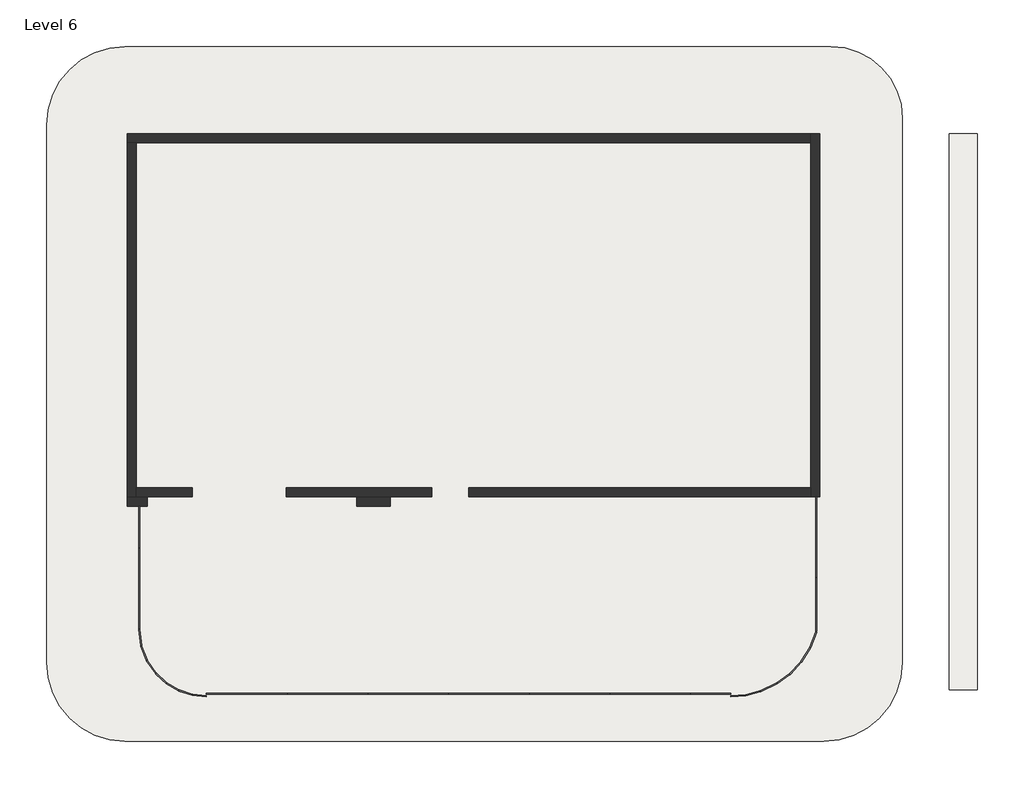
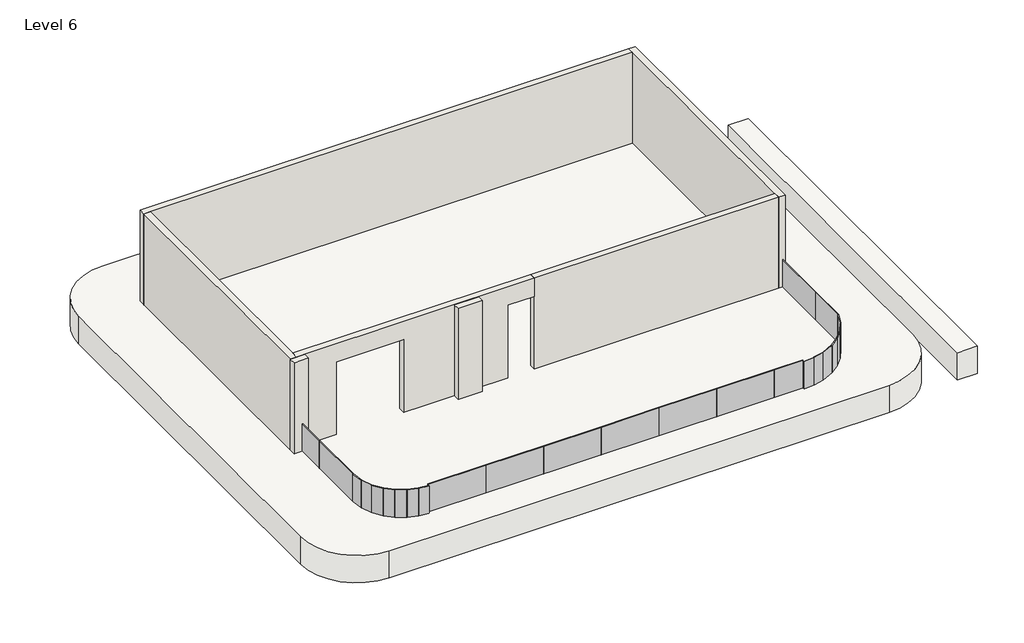
# One storey: 25 plates, 7 walls, 2 slabs.
"""IFC4 building model written with IfcOpenShell, lengths in millimetres."""

from ifc_helpers import new_model, si_unit, point, frame, frame_2d, origin, place, context, project, spatial, polyline, circle_curve, trimmed, segment, composite_curve, outline, extrude, faceted_brep, transform, mapped, element, save
from components import system_panel_glazed_95be5de7, system_panel_glazed_8746fe8c, system_panel_glazed_70ef586e, system_panel_glazed_2e848b93, system_panel_glazed_d6f392a9, system_panel_glazed_76d2efde, system_panel_glazed_1eaf0385, system_panel_glazed_cfef7f4a, system_panel_glazed_abbe3f8f, system_panel_glazed_0a91d840, system_panel_glazed_0f72cd4c, system_panel_glazed_404bb2e9, system_panel_glazed_ab35909a, system_panel_glazed_299ce7ab

model = new_model("IFC4")

# Units and contexts
model_context = context("Model", 3, world=origin())
ifc_project = project(units=[si_unit("LENGTHUNIT", "METRE", prefix="MILLI")], contexts=[model_context])

# Site, building, storey
site = spatial("IfcSite", under=ifc_project)
building = spatial("IfcBuilding", under=site)
storey = spatial("IfcBuildingStorey", under=building, Name="Level 6", Elevation=15240.0)

# Plates
placement = place(None, origin())
system_panel_glazed_shape = system_panel_glazed_95be5de7(model_context)
element("IfcPlate", 1, ObjectType="System Panel : Glazed", at=placement, inside=storey, context=model_context, shape_type="MappedRepresentation", body=[
    mapped(system_panel_glazed_shape, transform((-116.9533244, 3328.5792748, 15862.3), x_axis=(0.0, -1.0, 0.0), y_axis=(1.0, 0.0, 0.0), z_axis=(0.0, 0.0, 1.0))),
])
element("IfcPlate", 2, ObjectType="System Panel : Glazed", at=placement, inside=storey, context=model_context, shape_type="MappedRepresentation", body=[
    mapped(system_panel_glazed_shape, transform((-15410.278953, 2160.0432662, 15862.3), x_axis=(0.0, 1.0, 0.0), y_axis=(-1.0, 0.0, 0.0), z_axis=(0.0, 0.0, 1.0))),
])
system_panel_glazed_2_shape = system_panel_glazed_8746fe8c(model_context)
element("IfcPlate", 3, ObjectType="System Panel : Glazed", at=placement, inside=storey, context=model_context, shape_type="MappedRepresentation", body=[
    mapped(system_panel_glazed_2_shape, transform((-15386.0907484, 1056.9948552, 15862.3), x_axis=(-0.12717730440498623, 0.9918799994174101, 0.0), y_axis=(-0.9918799994174101, -0.12717730440498623, 0.0), z_axis=(0.0, 0.0, 1.0))),
])
system_panel_glazed_3_shape = system_panel_glazed_70ef586e(model_context)
element("IfcPlate", 4, ObjectType="System Panel : Glazed", at=placement, inside=storey, context=model_context, shape_type="MappedRepresentation", body=[
    mapped(system_panel_glazed_3_shape, transform((-15300.9211317, 710.4162823, 15862.3), x_axis=(-0.36020879862792143, 0.9328717068230924, 0.0), y_axis=(-0.9328717068230924, -0.36020879862792143, 0.0), z_axis=(0.0, 0.0, 1.0))),
])
system_panel_glazed_4_shape = system_panel_glazed_2e848b93(model_context)
element("IfcPlate", 5, ObjectType="System Panel : Glazed", at=placement, inside=storey, context=model_context, shape_type="MappedRepresentation", body=[
    mapped(system_panel_glazed_4_shape, transform((-15136.4134084, 402.4891221, 15862.3), x_axis=(-0.5680307758785693, 0.8230073132450225, 0.0), y_axis=(-0.8230073132450225, -0.5680307758785693, 0.0), z_axis=(0.0, 0.0, 1.0))),
])
system_panel_glazed_5_shape = system_panel_glazed_d6f392a9(model_context)
element("IfcPlate", 6, ObjectType="System Panel : Glazed", at=placement, inside=storey, context=model_context, shape_type="MappedRepresentation", body=[
    mapped(system_panel_glazed_5_shape, transform((-14917.4266334, 147.1103352, 15862.3), x_axis=(-0.7386085467399861, 0.6741345671916296, 0.0), y_axis=(-0.6741345671916296, -0.7386085467399861, 0.0), z_axis=(0.0, 0.0, 1.0))),
])
system_panel_glazed_6_shape = system_panel_glazed_76d2efde(model_context)
element("IfcPlate", 7, ObjectType="System Panel : Glazed", at=placement, inside=storey, context=model_context, shape_type="MappedRepresentation", body=[
    mapped(system_panel_glazed_6_shape, transform((-14071.8974005, -233.1578788, 15862.3), x_axis=(-0.994403599652405, 0.10564791052519545, 0.0), y_axis=(-0.10564791052519545, -0.994403599652405, 0.0), z_axis=(0.0, 0.0, 1.0))),
])
element("IfcPlate", 8, ObjectType="System Panel : Glazed", at=placement, inside=storey, context=model_context, shape_type="MappedRepresentation", body=[
    mapped(system_panel_glazed_6_shape, transform((-14665.5846616, -38.0381812, 15862.3), x_axis=(-0.8631975005225224, 0.5048663933078434, 0.0), y_axis=(-0.5048663933078434, -0.8631975005225224, 0.0), z_axis=(0.0, 0.0, 1.0))),
])
element("IfcPlate", 9, ObjectType="System Panel : Glazed", at=placement, inside=storey, context=model_context, shape_type="MappedRepresentation", body=[
    mapped(system_panel_glazed_6_shape, transform((-14379.1060319, -167.1354353, 15862.3), x_axis=(-0.9500075321236097, 0.31222698299219553, 0.0), y_axis=(-0.31222698299219553, -0.9500075321236097, 0.0), z_axis=(0.0, 0.0, 1.0))),
])
system_panel_glazed_7_shape = system_panel_glazed_1eaf0385(model_context)
element("IfcPlate", 10, ObjectType="System Panel : Glazed", at=placement, inside=storey, context=model_context, shape_type="MappedRepresentation", body=[
    mapped(system_panel_glazed_7_shape, transform((-15410.278953, 3550.7612705, 15862.3), x_axis=(0.0, 1.0, 0.0), y_axis=(-1.0, 0.0, 0.0), z_axis=(0.0, 0.0, 1.0))),
])
system_panel_glazed_8_shape = system_panel_glazed_cfef7f4a(model_context)
element("IfcPlate", 11, ObjectType="System Panel : Glazed", at=placement, inside=storey, context=model_context, shape_type="MappedRepresentation", body=[
    mapped(system_panel_glazed_8_shape, transform((-116.9533244, 1804.5112705, 15862.3), x_axis=(0.0, -1.0, 0.0), y_axis=(1.0, 0.0, 0.0), z_axis=(0.0, 0.0, 1.0))),
])
system_panel_glazed_9_shape = system_panel_glazed_abbe3f8f(model_context)
element("IfcPlate", 12, ObjectType="System Panel : Glazed", at=placement, inside=storey, context=model_context, shape_type="MappedRepresentation", body=[
    mapped(system_panel_glazed_9_shape, transform((-13000.3858906, -249.8497962, 15855.95), x_axis=(1.0, 0.0, 0.0), y_axis=(0.0, 1.0, 0.0), z_axis=(0.0, 0.0, 1.0))),
])
element("IfcPlate", 13, ObjectType="System Panel : Glazed", at=placement, inside=storey, context=model_context, shape_type="MappedRepresentation", body=[
    mapped(system_panel_glazed_9_shape, transform((-11171.5858906, -249.8497962, 15855.95), x_axis=(1.0, 0.0, 0.0), y_axis=(0.0, 1.0, 0.0), z_axis=(0.0, 0.0, 1.0))),
])
element("IfcPlate", 14, ObjectType="System Panel : Glazed", at=placement, inside=storey, context=model_context, shape_type="MappedRepresentation", body=[
    mapped(system_panel_glazed_9_shape, transform((-9342.7858906, -249.8497962, 15855.95), x_axis=(1.0, 0.0, 0.0), y_axis=(0.0, 1.0, 0.0), z_axis=(0.0, 0.0, 1.0))),
])
element("IfcPlate", 15, ObjectType="System Panel : Glazed", at=placement, inside=storey, context=model_context, shape_type="MappedRepresentation", body=[
    mapped(system_panel_glazed_9_shape, transform((-7513.9858906, -249.8497962, 15855.95), x_axis=(1.0, 0.0, 0.0), y_axis=(0.0, 1.0, 0.0), z_axis=(0.0, 0.0, 1.0))),
])
element("IfcPlate", 16, ObjectType="System Panel : Glazed", at=placement, inside=storey, context=model_context, shape_type="MappedRepresentation", body=[
    mapped(system_panel_glazed_9_shape, transform((-5685.1858906, -249.8497962, 15855.95), x_axis=(1.0, 0.0, 0.0), y_axis=(0.0, 1.0, 0.0), z_axis=(0.0, 0.0, 1.0))),
])
element("IfcPlate", 17, ObjectType="System Panel : Glazed", at=placement, inside=storey, context=model_context, shape_type="MappedRepresentation", body=[
    mapped(system_panel_glazed_9_shape, transform((-3856.3858906, -249.8497962, 15855.95), x_axis=(1.0, 0.0, 0.0), y_axis=(0.0, 1.0, 0.0), z_axis=(0.0, 0.0, 1.0))),
])
system_panel_glazed_10_shape = system_panel_glazed_0a91d840(model_context)
element("IfcPlate", 18, ObjectType="System Panel : Glazed", at=placement, inside=storey, context=model_context, shape_type="MappedRepresentation", body=[
    mapped(system_panel_glazed_10_shape, transform((-2484.7858906, -249.8497962, 15855.95), x_axis=(1.0, 0.0, 0.0), y_axis=(0.0, 1.0, 0.0), z_axis=(0.0, 0.0, 1.0))),
])
system_panel_glazed_11_shape = system_panel_glazed_0f72cd4c(model_context)
element("IfcPlate", 19, ObjectType="System Panel : Glazed", at=placement, inside=storey, context=model_context, shape_type="MappedRepresentation", body=[
    mapped(system_panel_glazed_11_shape, transform((-1181.9624413, -48.7697426, 15855.95), x_axis=(-0.9036899876908312, -0.4281873493546319, 0.0), y_axis=(0.4281873493546319, -0.9036899876908312, 0.0), z_axis=(0.0, 0.0, 1.0))),
])
system_panel_glazed_12_shape = system_panel_glazed_404bb2e9(model_context)
element("IfcPlate", 20, ObjectType="System Panel : Glazed", at=placement, inside=storey, context=model_context, shape_type="MappedRepresentation", body=[
    mapped(system_panel_glazed_12_shape, transform((-854.9951193, 142.6972628, 15855.95), x_axis=(-0.8053846593635025, -0.5927525204180369, 0.0), y_axis=(0.5927525204180369, -0.8053846593635025, 0.0), z_axis=(0.0, 0.0, 1.0))),
])
system_panel_glazed_13_shape = system_panel_glazed_ab35909a(model_context)
element("IfcPlate", 21, ObjectType="System Panel : Glazed", at=placement, inside=storey, context=model_context, shape_type="MappedRepresentation", body=[
    mapped(system_panel_glazed_13_shape, transform((-185.6986412, 1018.3780736, 15855.95), x_axis=(-0.36299643103623197, -0.931790529601454, 0.0), y_axis=(0.931790529601454, -0.36299643103623197, 0.0), z_axis=(0.0, 0.0, 1.0))),
])
element("IfcPlate", 22, ObjectType="System Panel : Glazed", at=placement, inside=storey, context=model_context, shape_type="MappedRepresentation", body=[
    mapped(system_panel_glazed_13_shape, transform((-586.0254267, 383.396855, 15855.95), x_axis=(-0.6842264553506641, -0.7292696057002963, 0.0), y_axis=(0.7292696057002963, -0.6842264553506641, 0.0), z_axis=(0.0, 0.0, 1.0))),
])
element("IfcPlate", 23, ObjectType="System Panel : Glazed", at=placement, inside=storey, context=model_context, shape_type="MappedRepresentation", body=[
    mapped(system_panel_glazed_13_shape, transform((-355.4442972, 681.7104644, 15855.95), x_axis=(-0.53331287683458, -0.8459180666012662, 0.0), y_axis=(0.8459180666012662, -0.53331287683458, 0.0), z_axis=(0.0, 0.0, 1.0))),
])
system_panel_glazed_14_shape = system_panel_glazed_299ce7ab(model_context)
element("IfcPlate", 24, ObjectType="System Panel : Glazed", at=placement, inside=storey, context=model_context, shape_type="MappedRepresentation", body=[
    mapped(system_panel_glazed_14_shape, transform((-1531.6778563, -179.6234093, 15855.95), x_axis=(-0.968084530428735, -0.2506239053733216, 0.0), y_axis=(0.2506239053733216, -0.968084530428735, 0.0), z_axis=(0.0, 0.0, 1.0))),
])
element("IfcPlate", 25, ObjectType="System Panel : Glazed", at=placement, inside=storey, context=model_context, shape_type="MappedRepresentation", body=[
    mapped(system_panel_glazed_14_shape, transform((-1860.7003711, -235.7241331, 15855.95), x_axis=(-0.9964369295237279, -0.08434124424814608, 0.0), y_axis=(0.08434124424814608, -0.9964369295237279, 0.0), z_axis=(0.0, 0.0, 1.0))),
])

# Slabs
element("IfcSlab", 26, ObjectType="Generic - 3' black", at=placement, inside=storey, context=model_context, shape_type="SweptSolid", body=[
    extrude(outline(composite_curve([segment(trimmed(circle_curve(frame_2d((238.6466756, 12828.0432662)), 1625.6), [point((238.6466756, 14453.6432662))], [point((1864.2466756, 12828.0432662))], False, "CARTESIAN"), True, "CONTINUOUS"), segment(polyline([(1864.2466756, 12828.0432662), (1864.2466756, 483.6432662)]), True, "CONTINUOUS"), segment(trimmed(circle_curve(frame_2d((86.2466756, 483.6432662)), 1778.0), [point((1864.2466756, 483.6432662))], [point((86.2466756, -1294.3567338))], False, "CARTESIAN"), True, "CONTINUOUS"), segment(polyline([(86.2466756, -1294.3567338), (-15763.3533244, -1294.3567338)]), True, "CONTINUOUS"), segment(trimmed(circle_curve(frame_2d((-15763.3533244, 483.6432662)), 1778.0), [point((-15763.3533244, -1294.3567338))], [point((-17541.3533244, 483.6432662))], False, "CARTESIAN"), True, "CONTINUOUS"), segment(polyline([(-17541.3533244, 483.6432662), (-17541.3533244, 12675.6432662)]), True, "CONTINUOUS"), segment(trimmed(circle_curve(frame_2d((-15763.3533244, 12675.6432662)), 1778.0), [point((-17541.3533244, 12675.6432662))], [point((-15763.3533244, 14453.6432662))], False, "CARTESIAN"), True, "CONTINUOUS"), segment(polyline([(-15763.3533244, 14453.6432662), (238.6466756, 14453.6432662)]), True, "CONTINUOUS")], self_intersect=False)), frame((0.0, 0.0, 14941.55), z_axis=(0.0, 0.0, 1.0), x_axis=(1.0, 0.0, 0.0)), (0.0, 0.0, 1.0), 914.4),
])
element("IfcSlab", 27, ObjectType="Generic - 3' black", at=placement, inside=storey, context=model_context, shape_type="SweptSolid", body=[
    extrude(outline(polyline([(2931.0466756, 12472.5792748), (3566.0466756, 12472.5792748), (3566.0466756, -125.9567338), (2931.0466756, -125.9567338), (2931.0466756, 12472.5792748)])), frame((0.0, 0.0, 14325.6), z_axis=(0.0, 0.0, 1.0), x_axis=(1.0, 0.0, 0.0)), (0.0, 0.0, 1.0), 914.4),
])

# Walls
element("IfcWall", 28, ObjectType="Generic - 8\" brown", at=placement, inside=storey, context=model_context, shape_type="SweptSolid", body=[
    extrude(outline(polyline([(-15255.3533244, 4027.0792748), (-15712.5533244, 4027.0792748), (-15712.5533244, 4230.2792748), (-15255.3533244, 4230.2792748), (-15255.3533244, 4027.0792748)])), frame((0.0, 0.0, 15862.3), z_axis=(0.0, 0.0, 1.0), x_axis=(1.0, 0.0, 0.0)), (0.0, 0.0, 1.0), 3048.0),
])
element("IfcWall", 29, ObjectType="Generic - 8\" brown", at=placement, inside=storey, context=model_context, shape_type="SweptSolid", body=[
    extrude(outline(polyline([(-9743.5533244, 4027.0792748), (-10505.5533244, 4027.0792748), (-10505.5533244, 4230.2792748), (-9743.5533244, 4230.2792748), (-9743.5533244, 4027.0792748)])), frame((0.0, 0.0, 15862.3), z_axis=(0.0, 0.0, 1.0), x_axis=(1.0, 0.0, 0.0)), (0.0, 0.0, 1.0), 3048.0),
])
element("IfcWall", 30, ObjectType="Generic - 8\" wood", at=placement, inside=storey, context=model_context, shape_type="Brep", body=[
    faceted_brep([(-15712.5533244, 12269.3792748, 15862.3), (-15509.3533244, 12269.3792748, 15862.3), (-218.5533244, 12269.3792748, 15862.3), (-218.5533244, 12269.3792748, 18910.3), (-15509.3533244, 12269.3792748, 18910.3), (-15712.5533244, 12269.3792748, 18910.3), (-15712.5533244, 12472.5792748, 15862.3), (-15712.5533244, 12472.5792748, 18910.3), (-218.5533244, 12472.5792748, 18910.3), (-218.5533244, 12472.5792748, 15862.3)], [[[0, 1, 2, 3, 4, 5]], [[6, 7, 8, 9]], [[2, 1, 0, 6, 9]], [[5, 4, 3, 8, 7]], [[0, 5, 7, 6]], [[3, 2, 9, 8]]]),
])
element("IfcWall", 31, ObjectType="Generic - 8\" wood", at=placement, inside=storey, context=model_context, shape_type="Brep", body=[
    faceted_brep([(-15509.3533244, 4242.9792748, 15862.3), (-15509.3533244, 4446.1792748, 15862.3), (-15509.3533244, 12269.3792748, 15862.3), (-15509.3533244, 12269.3792748, 18910.3), (-15509.3533244, 4446.1792748, 18910.3), (-15509.3533244, 4242.9792748, 18910.3), (-15712.5533244, 4242.9792748, 15862.3), (-15712.5533244, 4242.9792748, 18910.3), (-15712.5533244, 12269.3792748, 18910.3), (-15712.5533244, 12269.3792748, 15862.3)], [[[0, 1, 2, 3, 4, 5]], [[6, 7, 8, 9]], [[2, 1, 0, 6, 9]], [[5, 4, 3, 8, 7]], [[0, 5, 7, 6]], [[3, 2, 9, 8]]]),
])
element("IfcWall", 32, ObjectType="Generic - 8\" wood", at=placement, inside=storey, context=model_context, shape_type="Brep", body=[
    faceted_brep([(-218.5533244, 12472.5792748, 15862.3), (-218.5533244, 12269.3792748, 15862.3), (-218.5533244, 4446.1792748, 15862.3), (-218.5533244, 4242.9792748, 15862.3), (-218.5533244, 4242.9792748, 18910.3), (-218.5533244, 4446.1792748, 18910.3), (-218.5533244, 12269.3792748, 18910.3), (-218.5533244, 12472.5792748, 18910.3), (-15.3533244, 12472.5792748, 15862.3), (-15.3533244, 12472.5792748, 18910.3), (-15.3533244, 4242.9792748, 18910.3), (-15.3533244, 4242.9792748, 15862.3)], [[[0, 1, 2, 3, 4, 5, 6, 7]], [[8, 9, 10, 11]], [[3, 2, 1, 0, 8, 11]], [[7, 6, 5, 4, 10, 9]], [[0, 7, 9, 8]], [[4, 3, 11, 10]]]),
])
element("IfcWall", 33, ObjectType="Generic - 8\" wood", at=placement, inside=storey, context=model_context, shape_type="SweptSolid", body=[
    extrude(outline(polyline([(15862.3, -15509.3533244), (15862.3, -14243.2931037), (18300.7, -14243.2931037), (18300.7, -12109.6931037), (15862.3, -12109.6931037), (15862.3, -8802.0384076), (18300.7, -8802.0384076), (18300.7, -7965.5533244), (18910.3, -7965.5533244), (18910.3, -15509.3533244), (15862.3, -15509.3533244)])), frame((0.0, 4242.9792748, 0.0), z_axis=(0.0, 1.0, 0.0), x_axis=(0.0, 0.0, 1.0)), (0.0, 0.0, 1.0), 203.2),
])
element("IfcWall", 34, ObjectType="Generic - 8\" wood 2", at=placement, inside=storey, context=model_context, shape_type="SweptSolid", body=[
    extrude(outline(polyline([(-7965.5533244, 4446.1792748), (-218.5533244, 4446.1792748), (-218.5533244, 4242.9792748), (-7965.5533244, 4242.9792748), (-7965.5533244, 4446.1792748)])), frame((0.0, 0.0, 15862.3), z_axis=(0.0, 0.0, 1.0), x_axis=(1.0, 0.0, 0.0)), (0.0, 0.0, 1.0), 3048.0),
])

save(model, "model.ifc")

# Revit data of these elements
# Type "System Panel : Glazed"
#   Construction Type Id = "GSP4R"
#   Analytic Construction = "1/8 in Pilkington single glazing"
#   Visual Light Transmittance = 0.9
#   Solar Heat Gain Coefficient = 0.86
#   Heat Transfer Coefficient (U) = 1.18115 BTU/(h·ft²·°F)
# Type "Generic - 3' black"
#   Assembly Code = "B1010"
#   Function = 0
#   Layers, outside or top first: 3' - 0" "Door - Frame" (function 1)
# Type "Generic - 8\" brown"
#   Assembly Code = "B2010"
#   Layers, outside or top first: 0' - 8" "Door - Panel" (function 1)
# Type "Generic - 8\" wood"
#   Assembly Code = "B2010"
#   Layers, outside or top first: 0' - 8" "Cherry" (function 1)
# Type "Generic - 8\" wood 2"
#   Assembly Code = "B2010"
#   Layers, outside or top first: 0' - 8" "Concrete, Precast" (function 1)
# Elements 1, 2, 3, 4, 5, 6, 7, 8, 9, 10, 11, 12, 13, 14, 15, 16, 17, 18, 19, 20, 21, 22, 23, 24, 25 (IfcPlate, "System Panel : Glazed")
#   Phase Created = New Construction
#   Materials on its faces: "Glass"
# Element 26 (IfcSlab, "Generic - 3' black")
#   Height Offset From Level = 2' - 0 1/4"
#   Phase Created = New Construction
#   Materials on its faces: "Door - Frame"
# Element 27 (IfcSlab, "Generic - 3' black")
#   built-in parameter 1001955 = 3.14159 (stored number, unit not read)
#   Height Offset From Level = 0' - 0"
#   Phase Created = New Construction
#   Materials on its faces: "Door - Frame"
# Elements 28, 29 (IfcWall, "Generic - 8\" brown")
#   built-in parameter 1001111 = 2' - 0 1/2"
#   Top Offset = 0' - 0"
#   Base Offset = 2' - 0 1/2"
#   Unconnected Height = 10' - 0"
#   wall height = 10' - 0"
#   Phase Created = New Construction
#   Base Constraint = Level 6
#   Materials on its faces: "Door - Panel"
# Elements 30, 31, 33 (IfcWall, "Generic - 8\" wood")
#   built-in parameter 1001111 = 2' - 0 1/2"
#   Top Offset = 0' - 0"
#   Base Offset = 2' - 0 1/2"
#   Unconnected Height = 10' - 0"
#   wall height = 10' - 0"
#   Phase Created = New Construction
#   Base Constraint = Level 6
#   Materials on its faces: "Cherry"
# Element 32 (IfcWall, "Generic - 8\" wood")
#   built-in parameter 1001111 = 2' - 0 1/2"
#   Top Offset = 0' - 0"
#   Base Offset = 2' - 0 1/2"
#   Unconnected Height = 10' - 0"
#   wall height = 10' - 0"
#   Phase Created = New Construction
#   Base Constraint = Level 6
#   Materials on its faces: "Cherry", "Concrete, Precast"
# Element 34 (IfcWall, "Generic - 8\" wood 2")
#   built-in parameter 1001111 = 2' - 0 1/2"
#   Top Offset = 0' - 0"
#   Base Offset = 2' - 0 1/2"
#   Unconnected Height = 10' - 0"
#   wall height = 10' - 0"
#   Phase Created = New Construction
#   Base Constraint = Level 6
#   Materials on its faces: "Concrete, Precast"
# Materials
#   "Door - Frame": colour RGB 118 70 51, transparency 0, Cost = 0
#   "Door - Panel": class "Wood", colour RGB 210 159 95, transparency 0, Cost = 0
#   "Cherry": class "Wood", colour RGB 238 208 179, transparency 0, Description = "Prunus Serotina", Cost = 0
#   "Concrete, Precast": class "Concrete", colour RGB 198 187 187, transparency 0, Description = "Precast concrete", Cost = 0
#   "Glass": class "Glass", colour RGB 0 128 192, transparency 0.75, Description = "Soda Lime Glass", Cost = 0
